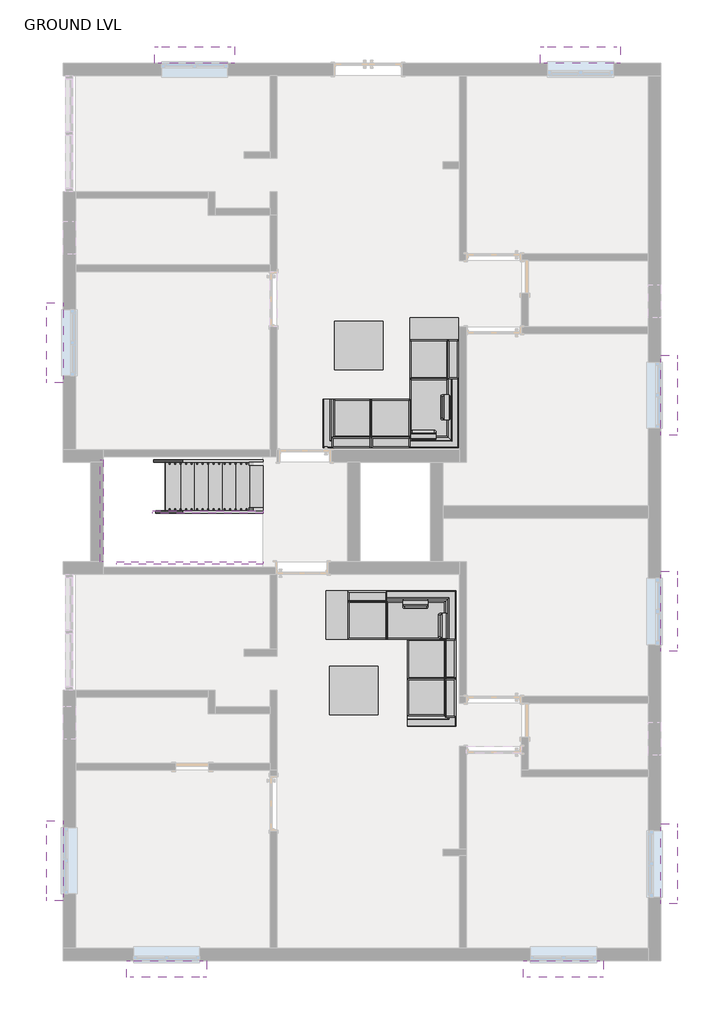
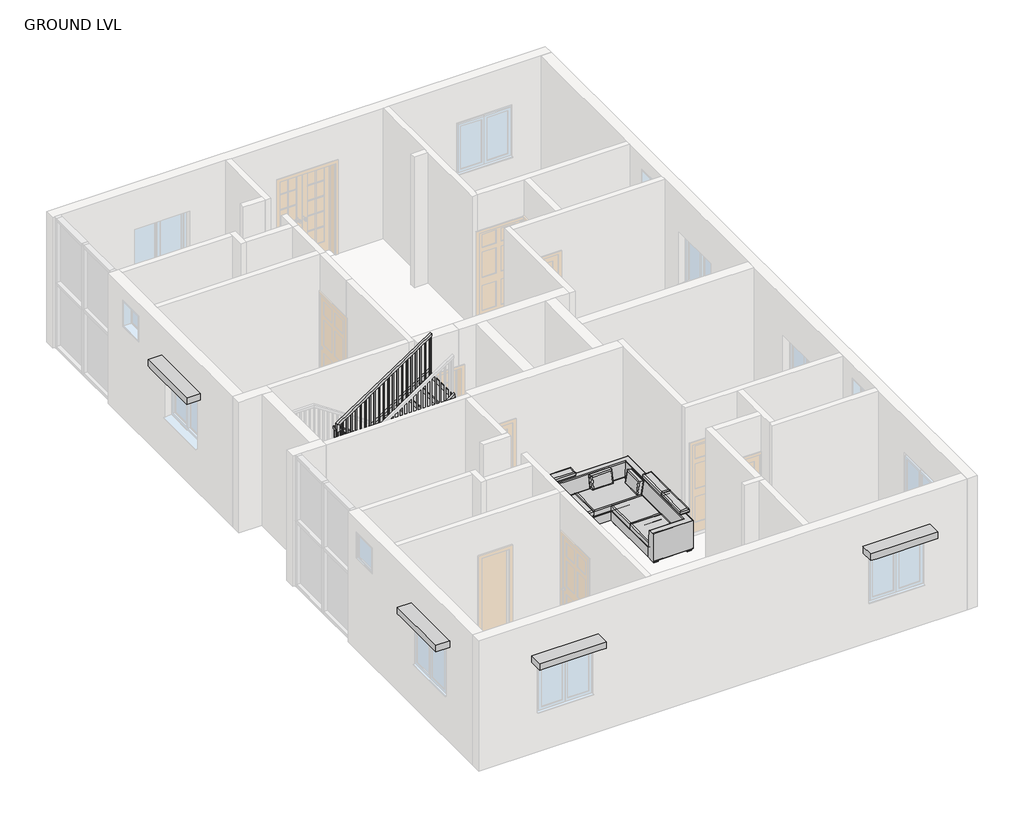
# One storey, part 4 of 4: 11 proxies, 5 members, 1 railing, 1 stair flight.
"""IFC4 building model written with IfcOpenShell, lengths in millimetres."""

from ifc_helpers import new_model, si_unit, frame, origin, place, context, project, spatial, polyline, outline, extrude, faceted_brep, transform, mapped, element, save
from components import generic_models_1_generic_models_1_fbb7ad13, generic_models_11_generic_models_11_d301a5e8, generic_models_21_generic_models_21_87948dc1, generic_models_36_generic_models_36_9c63594f, sectional_sofa_6482_sectional_sofa_6482_559db2f0, sectional_sofa_6482_sectional_sofa_6482_9496661e, stair_flight_80fd211d

model = new_model("IFC4")

# Units and contexts
model_context = context("Model", 3, world=origin())
ifc_project = project(units=[si_unit("LENGTHUNIT", "METRE", prefix="MILLI")], contexts=[model_context])

# Site, building, storey
site = spatial("IfcSite", under=ifc_project)
building = spatial("IfcBuilding", under=site)
storey = spatial("IfcBuildingStorey", under=building, Name="GROUND LVL", Elevation=3048.0)

# Proxies
placement = place(None, origin())
generic_models_1_generic_models_1_shape = generic_models_1_generic_models_1_fbb7ad13(model_context)
element("IfcBuildingElementProxy", 1, Name="Generic Models 10 : Generic Models 1", ObjectType="Generic Models 10 : Generic Models 1", at=placement, inside=storey, context=model_context, shape_type="MappedRepresentation", body=[
    mapped(generic_models_1_generic_models_1_shape, transform((7304.0875, 0.0, -12192.0), x_axis=(1.0, 0.0, 0.0), y_axis=(0.0, 1.0, 0.0), z_axis=(0.0, 0.0, 1.0))),
])
generic_models_11_generic_models_11_shape = generic_models_11_generic_models_11_d301a5e8(model_context)
element("IfcBuildingElementProxy", 2, Name="Generic Models 19 : Generic Models 11", ObjectType="Generic Models 19 : Generic Models 11", at=placement, inside=storey, context=model_context, shape_type="MappedRepresentation", body=[
    mapped(generic_models_11_generic_models_11_shape, transform((0.0, 0.0, -12192.0), x_axis=(1.0, 0.0, 0.0), y_axis=(0.0, 1.0, 0.0), z_axis=(0.0, 0.0, 1.0))),
])
element("IfcBuildingElementProxy", 3, Name="Generic Models 20 : Generic Models 11", ObjectType="Generic Models 20 : Generic Models 11", at=placement, inside=storey, context=model_context, shape_type="MappedRepresentation", body=[
    mapped(generic_models_11_generic_models_11_shape, transform((-7101.0359618, 0.0, -12192.0), x_axis=(1.0, 0.0, 0.0), y_axis=(0.0, 1.0, 0.0), z_axis=(0.0, 0.0, 1.0))),
])
generic_models_21_generic_models_21_shape = generic_models_21_generic_models_21_87948dc1(model_context)
element("IfcBuildingElementProxy", 4, Name="Generic Models 33 : Generic Models 21", ObjectType="Generic Models 33 : Generic Models 21", at=placement, inside=storey, context=model_context, shape_type="MappedRepresentation", body=[
    mapped(generic_models_21_generic_models_21_shape, transform((0.0, 0.0, -12192.0), x_axis=(1.0, 0.0, 0.0), y_axis=(0.0, 1.0, 0.0), z_axis=(0.0, 0.0, 1.0))),
])
element("IfcBuildingElementProxy", 5, Name="Generic Models 34 : Generic Models 21", ObjectType="Generic Models 34 : Generic Models 21", at=placement, inside=storey, context=model_context, shape_type="MappedRepresentation", body=[
    mapped(generic_models_21_generic_models_21_shape, transform((0.0, 4641.85, -12277.6), x_axis=(1.0, 0.0, 0.0), y_axis=(0.0, 1.0, 0.0), z_axis=(0.0, 0.0, 1.0))),
])
element("IfcBuildingElementProxy", 6, Name="Generic Models 35 : Generic Models 21", ObjectType="Generic Models 35 : Generic Models 21", at=placement, inside=storey, context=model_context, shape_type="MappedRepresentation", body=[
    mapped(generic_models_21_generic_models_21_shape, transform((0.0, 8616.95, -12277.6), x_axis=(1.0, 0.0, 0.0), y_axis=(0.0, 1.0, 0.0), z_axis=(0.0, 0.0, 1.0))),
])
generic_models_36_generic_models_36_shape = generic_models_36_generic_models_36_9c63594f(model_context)
element("IfcBuildingElementProxy", 7, Name="Generic Models 44 : Generic Models 36", ObjectType="Generic Models 44 : Generic Models 36", at=placement, inside=storey, context=model_context, shape_type="MappedRepresentation", body=[
    mapped(generic_models_36_generic_models_36_shape, transform((0.0, 0.0, -12192.0), x_axis=(1.0, 0.0, 0.0), y_axis=(0.0, 1.0, 0.0), z_axis=(0.0, 0.0, 1.0))),
])
element("IfcBuildingElementProxy", 8, Name="Generic Models 45 : Generic Models 36", ObjectType="Generic Models 45 : Generic Models 36", at=placement, inside=storey, context=model_context, shape_type="MappedRepresentation", body=[
    mapped(generic_models_36_generic_models_36_shape, transform((0.0, -9525.0, -12192.0), x_axis=(1.0, 0.0, 0.0), y_axis=(0.0, 1.0, 0.0), z_axis=(0.0, 0.0, 1.0))),
])
element("IfcBuildingElementProxy", 9, Name="Generic Models 9 : Generic Models 1", ObjectType="Generic Models 9 : Generic Models 1", at=placement, inside=storey, context=model_context, shape_type="MappedRepresentation", body=[
    mapped(generic_models_1_generic_models_1_shape, transform((0.0, 0.0, -12192.0), x_axis=(1.0, 0.0, 0.0), y_axis=(0.0, 1.0, 0.0), z_axis=(0.0, 0.0, 1.0))),
])
sectional_sofa_6482_sectional_sofa_6482_shape = sectional_sofa_6482_sectional_sofa_6482_559db2f0(model_context)
sectional_sofa_6482_sectional_sofa_6482_2_shape = sectional_sofa_6482_sectional_sofa_6482_9496661e(model_context)
element("IfcBuildingElementProxy", 10, Name="sectional_sofa_6482 : sectional_sofa_6482", ObjectType="sectional_sofa_6482 : sectional_sofa_6482", at=placement, inside=storey, context=model_context, shape_type="MappedRepresentation", body=[
    mapped(sectional_sofa_6482_sectional_sofa_6482_shape, transform((-474.7012202, 2273.0309003, 3048.0), x_axis=(1.0, 0.0, 0.0), y_axis=(0.0, 1.0, 0.0), z_axis=(0.0, 0.0, 1.0))),
    mapped(sectional_sofa_6482_sectional_sofa_6482_2_shape, transform((-474.7012202, 2273.0309003, 3048.0), x_axis=(1.0, 0.0, 0.0), y_axis=(0.0, 1.0, 0.0), z_axis=(0.0, 0.0, 1.0))),
])
element("IfcBuildingElementProxy", 11, Name="sectional_sofa_6482 : sectional_sofa_6482", ObjectType="sectional_sofa_6482 : sectional_sofa_6482", at=placement, inside=storey, context=model_context, shape_type="MappedRepresentation", body=[
    mapped(sectional_sofa_6482_sectional_sofa_6482_shape, transform((-449.3012202, 7467.3309003, 3048.0), x_axis=(0.0, -1.0, 0.0), y_axis=(1.0, 0.0, 0.0), z_axis=(0.0, 0.0, 1.0))),
    mapped(sectional_sofa_6482_sectional_sofa_6482_2_shape, transform((-449.3012202, 7467.3309003, 3048.0), x_axis=(0.0, -1.0, 0.0), y_axis=(1.0, 0.0, 0.0), z_axis=(0.0, 0.0, 1.0))),
])

# Members
element("IfcMember", 12, ObjectType="Stringer - 2\" Width", at=placement, inside=storey, context=model_context, shape_type="SweptSolid", body=[
    extrude(outline(polyline([(3048.0, -2748.0012202), (3266.0398409, -2748.0012202), (4586.8398409, -4729.2012202), (4220.5158313, -4729.2012202), (3048.0, -2970.4274732), (3048.0, -2748.0012202)])), frame((0.0, 4990.8309003, 0.0), z_axis=(0.0, 1.0, 0.0), x_axis=(0.0, 0.0, 1.0)), (0.0, 0.0, 1.0), 50.8),
])
element("IfcMember", 13, ObjectType="Stringer - 2\" Width", at=placement, inside=storey, context=model_context, shape_type="SweptSolid", body=[
    extrude(outline(polyline([(4790.0398409, -4780.0012202), (4423.7158313, -4780.0012202), (5778.382498, -2748.0012202), (6144.7065076, -2748.0012202), (4790.0398409, -4780.0012202)])), frame((0.0, 4990.8309003, 0.0), z_axis=(0.0, 1.0, 0.0), x_axis=(0.0, 0.0, 1.0)), (0.0, 0.0, 1.0), 50.8),
])
element("IfcMember", 14, ObjectType="Stringer - 2\" Width", at=placement, inside=storey, context=model_context, shape_type="SweptSolid", body=[
    extrude(outline(polyline([(3048.0, -2748.0012202), (3266.0398409, -2748.0012202), (4648.2, -4821.2414588), (4648.2, -5370.7274732), (3048.0, -2970.4274732), (3048.0, -2748.0012202)])), frame((0.0, 5930.6309003, 0.0), z_axis=(0.0, 1.0, 0.0), x_axis=(0.0, 0.0, 1.0)), (0.0, 0.0, 1.0), 50.8),
])
element("IfcMember", 15, ObjectType="Stringer - 2\" Width", at=placement, inside=storey, context=model_context, shape_type="SweptSolid", body=[
    extrude(outline(polyline([(-5745.2012202, 5981.4309003), (-5694.4012202, 5981.4309003), (-5694.4012202, 4101.8309003), (-5745.2012202, 4101.8309003), (-5745.2012202, 5981.4309003)])), frame((0.0, 0.0, 4343.4), z_axis=(0.0, 0.0, 1.0), x_axis=(1.0, 0.0, 0.0)), (0.0, 0.0, 1.0), 304.8),
])
element("IfcMember", 16, ObjectType="Stringer - 2\" Width", at=placement, inside=storey, context=model_context, shape_type="SweptSolid", body=[
    extrude(outline(polyline([(4343.4, -4900.4749672), (5778.382498, -2748.0012202), (6144.7065076, -2748.0012202), (4343.4, -5449.9609815), (4343.4, -4900.4749672)])), frame((0.0, 4051.0309003, 0.0), z_axis=(0.0, 1.0, 0.0), x_axis=(0.0, 0.0, 1.0)), (0.0, 0.0, 1.0), 50.8),
])

# Railing
element("IfcRailing", 17, ObjectType="Handrail - Rectangular", at=placement, inside=storey, context=model_context, shape_type="SolidModel", body=[
    faceted_brep([(-2748.0012202, 5041.6309003, 4131.7333333), (-2748.0012202, 5041.6309003, 4070.6793317), (-2748.0012202, 5092.4309003, 4070.6793317), (-2748.0012202, 5092.4309003, 4131.7333333), (-4703.8012202, 5041.6309003, 5435.6), (-4754.6012202, 5041.6309003, 5408.4126651), (-4754.6012202, 5092.4309003, 5408.4126651), (-4703.8012202, 5092.4309003, 5435.6), (-4703.8012202, 5041.6309003, 5486.4), (-4754.6012202, 5041.6309003, 5435.6), (-4754.6012202, 5092.4309003, 5435.6), (-4703.8012202, 5092.4309003, 5486.4), (-4780.0012202, 5041.6309003, 5486.4), (-4780.0012202, 5041.6309003, 5435.6), (-4830.8012202, 5092.4309003, 5435.6), (-4830.8012202, 5092.4309003, 5486.4), (-4780.0012202, 4990.8309003, 5486.4), (-4830.8012202, 4990.8309003, 5486.4), (-4830.8012202, 4940.0309003, 5435.6), (-4780.0012202, 4940.0309003, 5435.6)], [[[0, 1, 2, 3]], [[1, 0, 4, 5]], [[2, 1, 5, 6]], [[3, 2, 6, 7]], [[0, 3, 7, 4]], [[5, 4, 8, 9]], [[6, 5, 9, 10]], [[7, 6, 10, 11]], [[4, 7, 11, 8]], [[9, 8, 12, 13]], [[10, 9, 13, 14]], [[11, 10, 14, 15]], [[8, 11, 15, 12]], [[16, 17, 18, 19]], [[13, 12, 16, 19]], [[14, 13, 19, 18]], [[15, 14, 18, 17]], [[12, 15, 17, 16]]]),
    faceted_brep([(-4780.0012202, 4990.8309003, 5486.4), (-4780.0012202, 4940.0309003, 5435.6), (-4830.8012202, 4940.0309003, 5435.6), (-4830.8012202, 4990.8309003, 5486.4), (-4780.0012202, 4990.8309003, 5594.6793317), (-4830.8012202, 4990.8309003, 5621.8666667), (-4830.8012202, 4940.0309003, 5621.8666667), (-4780.0012202, 4940.0309003, 5594.6793317)], [[[0, 1, 2, 3]], [[4, 5, 6, 7]], [[1, 0, 4, 7]], [[2, 1, 7, 6]], [[3, 2, 6, 5]], [[0, 3, 5, 4]]]),
    faceted_brep([(-4830.8012202, 4990.8309003, 5621.8666667), (-4780.0012202, 4990.8309003, 5594.6793317), (-4780.0012202, 4940.0309003, 5594.6793317), (-4830.8012202, 4940.0309003, 5621.8666667), (-2748.0012202, 4990.8309003, 7010.4), (-2748.0012202, 4940.0309003, 7010.4), (-2748.0012202, 4940.0309003, 6949.3459984), (-2748.0012202, 4990.8309003, 6949.3459984)], [[[0, 1, 2, 3]], [[4, 5, 6, 7]], [[1, 0, 4, 7]], [[2, 1, 7, 6]], [[3, 2, 6, 5]], [[0, 3, 5, 4]]]),
    extrude(outline(polyline([(6926.0626651, -2782.9262202), (5926.6666667, -2782.9262202), (5926.6666667, -2763.8762202), (6938.7626651, -2763.8762202), (6926.0626651, -2782.9262202)])), frame((0.0, 4955.9059003, 0.0), z_axis=(0.0, 1.0, 0.0), x_axis=(0.0, 0.0, 1.0)), (0.0, 0.0, 1.0), 19.05),
    extrude(outline(polyline([(6858.3293317, -2884.5262202), (5926.6666667, -2884.5262202), (5926.6666667, -2865.4762202), (6871.0293317, -2865.4762202), (6858.3293317, -2884.5262202)])), frame((0.0, 4955.9059003, 0.0), z_axis=(0.0, 1.0, 0.0), x_axis=(0.0, 0.0, 1.0)), (0.0, 0.0, 1.0), 19.05),
    extrude(outline(polyline([(6790.5959984, -2986.1262202), (5926.6666667, -2986.1262202), (5926.6666667, -2967.0762202), (6803.2959984, -2967.0762202), (6790.5959984, -2986.1262202)])), frame((0.0, 4955.9059003, 0.0), z_axis=(0.0, 1.0, 0.0), x_axis=(0.0, 0.0, 1.0)), (0.0, 0.0, 1.0), 19.05),
    extrude(outline(polyline([(6722.8626651, -3087.7262202), (5757.3333333, -3087.7262202), (5757.3333333, -3068.6762202), (6735.5626651, -3068.6762202), (6722.8626651, -3087.7262202)])), frame((0.0, 4955.9059003, 0.0), z_axis=(0.0, 1.0, 0.0), x_axis=(0.0, 0.0, 1.0)), (0.0, 0.0, 1.0), 19.05),
    extrude(outline(polyline([(6655.1293317, -3189.3262202), (5757.3333333, -3189.3262202), (5757.3333333, -3170.2762202), (6667.8293317, -3170.2762202), (6655.1293317, -3189.3262202)])), frame((0.0, 4955.9059003, 0.0), z_axis=(0.0, 1.0, 0.0), x_axis=(0.0, 0.0, 1.0)), (0.0, 0.0, 1.0), 19.05),
    extrude(outline(polyline([(6587.3959984, -3290.9262202), (5588.0, -3290.9262202), (5588.0, -3271.8762202), (6600.0959984, -3271.8762202), (6587.3959984, -3290.9262202)])), frame((0.0, 4955.9059003, 0.0), z_axis=(0.0, 1.0, 0.0), x_axis=(0.0, 0.0, 1.0)), (0.0, 0.0, 1.0), 19.05),
    extrude(outline(polyline([(6519.6626651, -3392.5262202), (5588.0, -3392.5262202), (5588.0, -3373.4762202), (6532.3626651, -3373.4762202), (6519.6626651, -3392.5262202)])), frame((0.0, 4955.9059003, 0.0), z_axis=(0.0, 1.0, 0.0), x_axis=(0.0, 0.0, 1.0)), (0.0, 0.0, 1.0), 19.05),
    extrude(outline(polyline([(6451.9293317, -3494.1262202), (5588.0, -3494.1262202), (5588.0, -3475.0762202), (6464.6293317, -3475.0762202), (6451.9293317, -3494.1262202)])), frame((0.0, 4955.9059003, 0.0), z_axis=(0.0, 1.0, 0.0), x_axis=(0.0, 0.0, 1.0)), (0.0, 0.0, 1.0), 19.05),
    extrude(outline(polyline([(6384.1959984, -3595.7262202), (5418.6666667, -3595.7262202), (5418.6666667, -3576.6762202), (6396.8959984, -3576.6762202), (6384.1959984, -3595.7262202)])), frame((0.0, 4955.9059003, 0.0), z_axis=(0.0, 1.0, 0.0), x_axis=(0.0, 0.0, 1.0)), (0.0, 0.0, 1.0), 19.05),
    extrude(outline(polyline([(6316.4626651, -3697.3262202), (5418.6666667, -3697.3262202), (5418.6666667, -3678.2762202), (6329.1626651, -3678.2762202), (6316.4626651, -3697.3262202)])), frame((0.0, 4955.9059003, 0.0), z_axis=(0.0, 1.0, 0.0), x_axis=(0.0, 0.0, 1.0)), (0.0, 0.0, 1.0), 19.05),
    extrude(outline(polyline([(6248.7293317, -3798.9262202), (5249.3333333, -3798.9262202), (5249.3333333, -3779.8762202), (6261.4293317, -3779.8762202), (6248.7293317, -3798.9262202)])), frame((0.0, 4955.9059003, 0.0), z_axis=(0.0, 1.0, 0.0), x_axis=(0.0, 0.0, 1.0)), (0.0, 0.0, 1.0), 19.05),
    extrude(outline(polyline([(6180.9959984, -3900.5262202), (5249.3333333, -3900.5262202), (5249.3333333, -3881.4762202), (6193.6959984, -3881.4762202), (6180.9959984, -3900.5262202)])), frame((0.0, 4955.9059003, 0.0), z_axis=(0.0, 1.0, 0.0), x_axis=(0.0, 0.0, 1.0)), (0.0, 0.0, 1.0), 19.05),
    extrude(outline(polyline([(6113.2626651, -4002.1262202), (5249.3333333, -4002.1262202), (5249.3333333, -3983.0762202), (6125.9626651, -3983.0762202), (6113.2626651, -4002.1262202)])), frame((0.0, 4955.9059003, 0.0), z_axis=(0.0, 1.0, 0.0), x_axis=(0.0, 0.0, 1.0)), (0.0, 0.0, 1.0), 19.05),
    extrude(outline(polyline([(6045.5293317, -4103.7262202), (5080.0, -4103.7262202), (5080.0, -4084.6762202), (6058.2293317, -4084.6762202), (6045.5293317, -4103.7262202)])), frame((0.0, 4955.9059003, 0.0), z_axis=(0.0, 1.0, 0.0), x_axis=(0.0, 0.0, 1.0)), (0.0, 0.0, 1.0), 19.05),
    extrude(outline(polyline([(5977.7959984, -4205.3262202), (5080.0, -4205.3262202), (5080.0, -4186.2762202), (5990.4959984, -4186.2762202), (5977.7959984, -4205.3262202)])), frame((0.0, 4955.9059003, 0.0), z_axis=(0.0, 1.0, 0.0), x_axis=(0.0, 0.0, 1.0)), (0.0, 0.0, 1.0), 19.05),
    extrude(outline(polyline([(5910.0626651, -4306.9262202), (4910.6666667, -4306.9262202), (4910.6666667, -4287.8762202), (5922.7626651, -4287.8762202), (5910.0626651, -4306.9262202)])), frame((0.0, 4955.9059003, 0.0), z_axis=(0.0, 1.0, 0.0), x_axis=(0.0, 0.0, 1.0)), (0.0, 0.0, 1.0), 19.05),
    extrude(outline(polyline([(5842.3293317, -4408.5262202), (4910.6666667, -4408.5262202), (4910.6666667, -4389.4762202), (5855.0293317, -4389.4762202), (5842.3293317, -4408.5262202)])), frame((0.0, 4955.9059003, 0.0), z_axis=(0.0, 1.0, 0.0), x_axis=(0.0, 0.0, 1.0)), (0.0, 0.0, 1.0), 19.05),
    extrude(outline(polyline([(5774.5959984, -4510.1262202), (4910.6666667, -4510.1262202), (4910.6666667, -4491.0762202), (5787.2959984, -4491.0762202), (5774.5959984, -4510.1262202)])), frame((0.0, 4955.9059003, 0.0), z_axis=(0.0, 1.0, 0.0), x_axis=(0.0, 0.0, 1.0)), (0.0, 0.0, 1.0), 19.05),
    extrude(outline(polyline([(5706.8626651, -4611.7262202), (4741.3333333, -4611.7262202), (4741.3333333, -4592.6762202), (5719.5626651, -4592.6762202), (5706.8626651, -4611.7262202)])), frame((0.0, 4955.9059003, 0.0), z_axis=(0.0, 1.0, 0.0), x_axis=(0.0, 0.0, 1.0)), (0.0, 0.0, 1.0), 19.05),
    extrude(outline(polyline([(5639.1293317, -4713.3262202), (4741.3333333, -4713.3262202), (4741.3333333, -4694.2762202), (5651.8293317, -4694.2762202), (5639.1293317, -4713.3262202)])), frame((0.0, 4955.9059003, 0.0), z_axis=(0.0, 1.0, 0.0), x_axis=(0.0, 0.0, 1.0)), (0.0, 0.0, 1.0), 19.05),
    extrude(outline(polyline([(-4770.4762202, 5057.5059003), (-4789.5262202, 5057.5059003), (-4789.5262202, 5076.5559003), (-4770.4762202, 5076.5559003), (-4770.4762202, 5057.5059003)])), frame((0.0, 0.0, 4572.0), z_axis=(0.0, 0.0, 1.0), x_axis=(1.0, 0.0, 0.0)), (0.0, 0.0, 1.0), 863.6),
    extrude(outline(polyline([(5363.9626651, -4687.9262202), (4402.6666667, -4687.9262202), (4402.6666667, -4668.8762202), (5351.2626651, -4668.8762202), (5363.9626651, -4687.9262202)])), frame((0.0, 5057.5059003, 0.0), z_axis=(0.0, 1.0, 0.0), x_axis=(0.0, 0.0, 1.0)), (0.0, 0.0, 1.0), 19.05),
    extrude(outline(polyline([(5296.2293317, -4586.3262202), (4402.6666667, -4586.3262202), (4402.6666667, -4567.2762202), (5283.5293317, -4567.2762202), (5296.2293317, -4586.3262202)])), frame((0.0, 5057.5059003, 0.0), z_axis=(0.0, 1.0, 0.0), x_axis=(0.0, 0.0, 1.0)), (0.0, 0.0, 1.0), 19.05),
    extrude(outline(polyline([(5228.4959984, -4484.7262202), (4233.3333333, -4484.7262202), (4233.3333333, -4465.6762202), (5215.7959984, -4465.6762202), (5228.4959984, -4484.7262202)])), frame((0.0, 5057.5059003, 0.0), z_axis=(0.0, 1.0, 0.0), x_axis=(0.0, 0.0, 1.0)), (0.0, 0.0, 1.0), 19.05),
    extrude(outline(polyline([(5160.7626651, -4383.1262202), (4233.3333333, -4383.1262202), (4233.3333333, -4364.0762202), (5148.0626651, -4364.0762202), (5160.7626651, -4383.1262202)])), frame((0.0, 5057.5059003, 0.0), z_axis=(0.0, 1.0, 0.0), x_axis=(0.0, 0.0, 1.0)), (0.0, 0.0, 1.0), 19.05),
    extrude(outline(polyline([(5093.0293317, -4281.5262202), (4233.3333333, -4281.5262202), (4233.3333333, -4262.4762202), (5080.3293317, -4262.4762202), (5093.0293317, -4281.5262202)])), frame((0.0, 5057.5059003, 0.0), z_axis=(0.0, 1.0, 0.0), x_axis=(0.0, 0.0, 1.0)), (0.0, 0.0, 1.0), 19.05),
    extrude(outline(polyline([(5025.2959984, -4179.9262202), (4064.0, -4179.9262202), (4064.0, -4160.8762202), (5012.5959984, -4160.8762202), (5025.2959984, -4179.9262202)])), frame((0.0, 5057.5059003, 0.0), z_axis=(0.0, 1.0, 0.0), x_axis=(0.0, 0.0, 1.0)), (0.0, 0.0, 1.0), 19.05),
    extrude(outline(polyline([(4957.5626651, -4078.3262202), (4064.0, -4078.3262202), (4064.0, -4059.2762202), (4944.8626651, -4059.2762202), (4957.5626651, -4078.3262202)])), frame((0.0, 5057.5059003, 0.0), z_axis=(0.0, 1.0, 0.0), x_axis=(0.0, 0.0, 1.0)), (0.0, 0.0, 1.0), 19.05),
    extrude(outline(polyline([(4889.8293317, -3976.7262202), (3894.6666667, -3976.7262202), (3894.6666667, -3957.6762202), (4877.1293317, -3957.6762202), (4889.8293317, -3976.7262202)])), frame((0.0, 5057.5059003, 0.0), z_axis=(0.0, 1.0, 0.0), x_axis=(0.0, 0.0, 1.0)), (0.0, 0.0, 1.0), 19.05),
    extrude(outline(polyline([(4822.0959984, -3875.1262202), (3894.6666667, -3875.1262202), (3894.6666667, -3856.0762202), (4809.3959984, -3856.0762202), (4822.0959984, -3875.1262202)])), frame((0.0, 5057.5059003, 0.0), z_axis=(0.0, 1.0, 0.0), x_axis=(0.0, 0.0, 1.0)), (0.0, 0.0, 1.0), 19.05),
    extrude(outline(polyline([(4754.3626651, -3773.5262202), (3894.6666667, -3773.5262202), (3894.6666667, -3754.4762202), (4741.6626651, -3754.4762202), (4754.3626651, -3773.5262202)])), frame((0.0, 5057.5059003, 0.0), z_axis=(0.0, 1.0, 0.0), x_axis=(0.0, 0.0, 1.0)), (0.0, 0.0, 1.0), 19.05),
    extrude(outline(polyline([(4686.6293317, -3671.9262202), (3725.3333333, -3671.9262202), (3725.3333333, -3652.8762202), (4673.9293317, -3652.8762202), (4686.6293317, -3671.9262202)])), frame((0.0, 5057.5059003, 0.0), z_axis=(0.0, 1.0, 0.0), x_axis=(0.0, 0.0, 1.0)), (0.0, 0.0, 1.0), 19.05),
    extrude(outline(polyline([(4618.8959984, -3570.3262202), (3725.3333333, -3570.3262202), (3725.3333333, -3551.2762202), (4606.1959984, -3551.2762202), (4618.8959984, -3570.3262202)])), frame((0.0, 5057.5059003, 0.0), z_axis=(0.0, 1.0, 0.0), x_axis=(0.0, 0.0, 1.0)), (0.0, 0.0, 1.0), 19.05),
    extrude(outline(polyline([(4551.1626651, -3468.7262202), (3556.0, -3468.7262202), (3556.0, -3449.6762202), (4538.4626651, -3449.6762202), (4551.1626651, -3468.7262202)])), frame((0.0, 5057.5059003, 0.0), z_axis=(0.0, 1.0, 0.0), x_axis=(0.0, 0.0, 1.0)), (0.0, 0.0, 1.0), 19.05),
    extrude(outline(polyline([(4483.4293317, -3367.1262202), (3556.0, -3367.1262202), (3556.0, -3348.0762202), (4470.7293317, -3348.0762202), (4483.4293317, -3367.1262202)])), frame((0.0, 5057.5059003, 0.0), z_axis=(0.0, 1.0, 0.0), x_axis=(0.0, 0.0, 1.0)), (0.0, 0.0, 1.0), 19.05),
    extrude(outline(polyline([(4415.6959984, -3265.5262202), (3556.0, -3265.5262202), (3556.0, -3246.4762202), (4402.9959984, -3246.4762202), (4415.6959984, -3265.5262202)])), frame((0.0, 5057.5059003, 0.0), z_axis=(0.0, 1.0, 0.0), x_axis=(0.0, 0.0, 1.0)), (0.0, 0.0, 1.0), 19.05),
    extrude(outline(polyline([(4347.9626651, -3163.9262202), (3386.6666667, -3163.9262202), (3386.6666667, -3144.8762202), (4335.2626651, -3144.8762202), (4347.9626651, -3163.9262202)])), frame((0.0, 5057.5059003, 0.0), z_axis=(0.0, 1.0, 0.0), x_axis=(0.0, 0.0, 1.0)), (0.0, 0.0, 1.0), 19.05),
    extrude(outline(polyline([(4280.2293317, -3062.3262202), (3386.6666667, -3062.3262202), (3386.6666667, -3043.2762202), (4267.5293317, -3043.2762202), (4280.2293317, -3062.3262202)])), frame((0.0, 5057.5059003, 0.0), z_axis=(0.0, 1.0, 0.0), x_axis=(0.0, 0.0, 1.0)), (0.0, 0.0, 1.0), 19.05),
    extrude(outline(polyline([(4212.4959984, -2960.7262202), (3217.3333333, -2960.7262202), (3217.3333333, -2941.6762202), (4199.7959984, -2941.6762202), (4212.4959984, -2960.7262202)])), frame((0.0, 5057.5059003, 0.0), z_axis=(0.0, 1.0, 0.0), x_axis=(0.0, 0.0, 1.0)), (0.0, 0.0, 1.0), 19.05),
    extrude(outline(polyline([(4144.7626651, -2859.1262202), (3217.3333333, -2859.1262202), (3217.3333333, -2840.0762202), (4132.0626651, -2840.0762202), (4144.7626651, -2859.1262202)])), frame((0.0, 5057.5059003, 0.0), z_axis=(0.0, 1.0, 0.0), x_axis=(0.0, 0.0, 1.0)), (0.0, 0.0, 1.0), 19.05),
    extrude(outline(polyline([(-4795.8762202, 4974.9559003), (-4795.8762202, 4955.9059003), (-4814.9262202, 4955.9059003), (-4814.9262202, 4974.9559003), (-4795.8762202, 4974.9559003)])), frame((0.0, 0.0, 4572.0), z_axis=(0.0, 0.0, 1.0), x_axis=(1.0, 0.0, 0.0)), (0.0, 0.0, 1.0), 863.6),
    extrude(outline(polyline([(-4795.8762202, 5057.5059003), (-4814.9262202, 5057.5059003), (-4814.9262202, 5076.5559003), (-4795.8762202, 5076.5559003), (-4795.8762202, 5057.5059003)])), frame((0.0, 0.0, 4572.0), z_axis=(0.0, 0.0, 1.0), x_axis=(1.0, 0.0, 0.0)), (0.0, 0.0, 1.0), 863.6),
    extrude(outline(polyline([(6936.6459984, -2767.0512202), (5926.6666667, -2767.0512202), (5926.6666667, -2748.0012202), (6949.3459984, -2748.0012202), (6936.6459984, -2767.0512202)])), frame((0.0, 4955.9059003, 0.0), z_axis=(0.0, 1.0, 0.0), x_axis=(0.0, 0.0, 1.0)), (0.0, 0.0, 1.0), 19.05),
    extrude(outline(polyline([(4083.3793317, -2767.0512202), (3217.3333333, -2767.0512202), (3217.3333333, -2748.0012202), (4070.6793317, -2748.0012202), (4083.3793317, -2767.0512202)])), frame((0.0, 5057.5059003, 0.0), z_axis=(0.0, 1.0, 0.0), x_axis=(0.0, 0.0, 1.0)), (0.0, 0.0, 1.0), 19.05),
])

# Stair flight
stair_flight_shape = stair_flight_80fd211d(model_context)
element("IfcStairFlight", 18, ObjectType="2\" Tread 1\" Nosing 1/4\" Riser", at=placement, inside=storey, context=model_context, shape_type="MappedRepresentation", body=[
    mapped(stair_flight_shape, transform((0.0, 0.0, 0.0), x_axis=(1.0, 0.0, 0.0), y_axis=(0.0, 1.0, 0.0), z_axis=(0.0, 0.0, 1.0))),
])

save(model, "model.ifc")

# Revit data of these elements
# Type "sectional_sofa_6482 : sectional_sofa_6482"
#   frame trim = frame trim
#   fabric = Fabric
#   Frame = frame
#   FABRIC 2 = fabric 2
#   Default Elevation = 0
# Type "Handrail - Rectangular"
#   Assembly Code = "C2010400"
#   built-in parameter 1008612 = 0.0416667 (stored number, unit not read)
#   built-in parameter 1008611 = 0.0416667 (stored number, unit not read)
#   built-in parameter 1008609 = 0.333333 (stored number, unit not read)
#   built-in parameter 1008604 = 0.166667 (stored number, unit not read)
#   built-in parameter 1008603 = 0.166667 (stored number, unit not read)
#   Railing Height = 3' - 0"
#   built-in parameter 1008630 = 2
#   built-in parameter 1008610 = 2
#   built-in parameter 1008618 = Baluster - Square : 3/4"
# Element 1 (IfcBuildingElementProxy, "Generic Models 10 : Generic Models 1")
#   Phase Created = New Construction
#   Materials on its faces: "white"
# Element 2 (IfcBuildingElementProxy, "Generic Models 19 : Generic Models 11")
#   Phase Created = New Construction
#   Materials on its faces: "white"
# Element 3 (IfcBuildingElementProxy, "Generic Models 20 : Generic Models 11")
#   Phase Created = New Construction
#   Materials on its faces: "white"
# Element 4 (IfcBuildingElementProxy, "Generic Models 33 : Generic Models 21")
#   Phase Created = New Construction
#   Materials on its faces: "white"
# Element 5 (IfcBuildingElementProxy, "Generic Models 34 : Generic Models 21")
#   Phase Created = New Construction
#   Materials on its faces: "white"
# Element 6 (IfcBuildingElementProxy, "Generic Models 35 : Generic Models 21")
#   Phase Created = New Construction
#   Materials on its faces: "white"
# Element 7 (IfcBuildingElementProxy, "Generic Models 44 : Generic Models 36")
#   Phase Created = New Construction
#   Materials on its faces: "white"
# Element 8 (IfcBuildingElementProxy, "Generic Models 45 : Generic Models 36")
#   Phase Created = New Construction
#   Materials on its faces: "white"
# Element 9 (IfcBuildingElementProxy, "Generic Models 9 : Generic Models 1")
#   Phase Created = New Construction
#   Materials on its faces: "white"
# Elements 10, 11 (IfcBuildingElementProxy, "sectional_sofa_6482 : sectional_sofa_6482")
#   Phase Created = New Construction
#   Materials on its faces: "frame trim", "Fabric", "fabric 2", "frame"
# Elements 12, 13, 14, 15, 16 (IfcMember, "Stringer - 2\" Width")
#   Phase Created = New Construction
# Element 17 (IfcRailing, "Handrail - Rectangular")
#   Phase Created = New Construction
# Element 18 (IfcStairFlight, "2\" Tread 1\" Nosing 1/4\" Riser")
#   Phase Created = New Construction
# Materials
#   "frame trim": class "Metal", colour RGB 182 182 182, transparency 0
#   "Fabric": class "Textile", colour RGB 120 120 120, transparency 0, Description = "Fabric, gray stripes", Cost = 0
#   "frame": class "Wood", colour RGB 71 38 7, transparency 0
#   "fabric 2": class "Fabric", colour RGB 128 0 0, transparency 0
#   "white": class "Generic", colour RGB 120 120 120, transparency 0, Cost = 0
